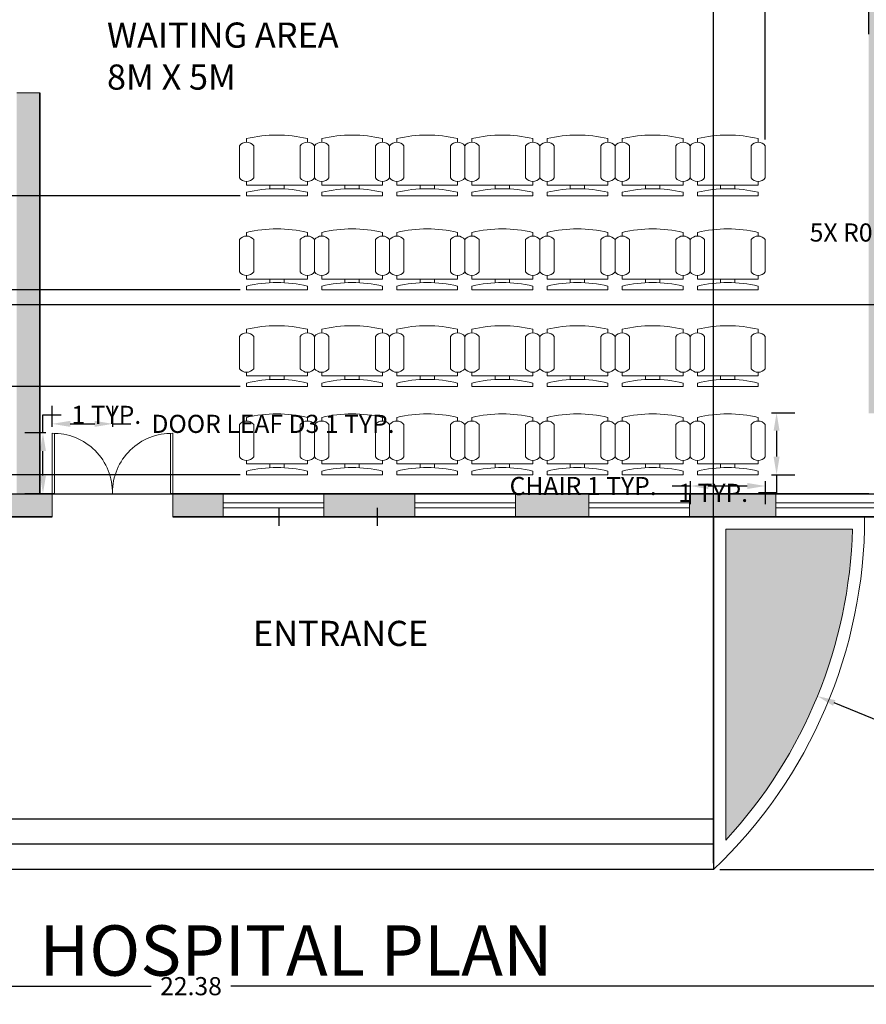
# Model space of a CAD drawing. Units: metres. Extents: x 4298.5 to 4325.2, y 2075 to 2095.8.
# Tile 20 of 35: x 4309.9 to 4318.3, y 2075 to 2084.8. Entities that reach past the tile are written whole.
import ezdxf

# ---------------------------------------------------------------- set-up
doc = ezdxf.new("R2010")
doc.units = ezdxf.units.M
for name, color, linetype, lineweight in [('A-ANNO-DIMS', 2, 'Continuous', 18), ('A-ANNO-TEXT', 7, 'Continuous', 25), ('A-AREA-IDEN', 7, 'Continuous', 18), ('A-DOOR', 3, 'Continuous', 18), ('A-FLOR-STRS', 7, 'Continuous', 25), ('A-FURN', 15, 'Continuous', 18), ('A-GLAZ', 4, 'Continuous', 18), ('A-WALL', 7, 'Continuous', 35), ('A-WALL-PATT', 252, 'Continuous', 13), ('L-PLNT-BEDS', 94, 'Continuous', 18), ('L-PLNT-BEDS-PATT', 252, 'Continuous', 13)]:
    doc.layers.add(name, color=color, linetype=linetype, lineweight=lineweight)
doc.styles.get("Standard").update_dxf_attribs({"font": 'arial.ttf'})
doc.dimstyles.get("Standard").update_dxf_attribs({"dimtxt": 0.18, "dimasz": 0.18, "dimexe": 0.18, "dimexo": 0.0625, "dimgap": 0.09, "dimtad": 0, "dimtih": 1, "dimtoh": 1, "dimdec": 4, "dimzin": 0, "dimdsep": 46, "dimtxsty": 'Standard', "dimcen": 0.09, "dimadec": 0, "dimazin": 0, "dimtfac": 1, "dimtdec": 4, "dimtofl": 0, "dimtmove": 0, "dimatfit": 3, "dimfxl": 1, "dimtolj": 1, "dimtzin": 0, "dimarcsym": 0})

# ---------------------------------------------------------------- blocks, each defined once
blk = doc.blocks.new('Chair - Desk')
for p, q in [((-8.5, 0), (-8.5, -1)), ((-8.5, 0), (8.5, 0)), ((8.5, 0), (8.5, -1)), ((-2, -3), (-2, -1.9355)), ((2, -1.9576), (2, -3)), ((-10.5, -5), (-10.5, -14)), ((-8.5, -3), (-8.5, -4)), ((-8.5, -3), (8.5, -3)), ((-6.5, -14), (-6.5, -5)), ((6.5, -5), (6.5, -14)), ((8.5, -3), (8.5, -4)), ((10.5, -14), (10.5, -5)), ((-8.5, -15), (-8.5, -16)), ((8.5, -15), (8.5, -16))]:
    blk.add_line(p, q)
for centre, radius, start, end in [((0, 34.625), 36.625, 256.5803, 283.4197), ((-8.5, -6.5), 2.5, 36.8699, 143.1301), ((8.5, -6.5), 2.5, 36.8699, 143.1301), ((-8.5, -12.5), 2.5, 216.8699, 323.1301), ((0, 19.625), 36.625, 256.5803, 283.4197), ((8.5, -12.5), 2.5, 216.8699, 323.1301)]:
    blk.add_arc(centre, radius, start, end)
blk = doc.blocks.new('WIN-1000-GLASS')
for p, q in [((1, 0.05), (0, 0.05)), ((1, 0), (0, 0))]:
    blk.add_line(p, q)
blk = doc.blocks.new('DOOR-600-LEAF')
for p, q in [((0, 0), (0, 0.6)), ((0.025, 0), (0.025, 0.6))]:
    blk.add_line(p, q)
blk.add_arc((0.0125, 0.0125), 0.5876, 358.78112, 91.21888)
blk = doc.blocks.new('*D19')
at = {"layer": 'A-ANNO-DIMS', "color": 0, "lineweight": -2, "transparency": 16777216}
for p, q in [((4316.5779, 2080.1351), (4316.3979, 2080.1351)), ((4316.5779, 2080.1845), (4316.5779, 2079.9551)), ((4317.144, 2080.1351), (4316.7579, 2080.1351)), ((4317.324, 2080.1845), (4317.324, 2079.9551))]:
    blk.add_line(p, q, dxfattribs=at)
at = {"layer": 'A-ANNO-DIMS', "color": 0, "transparency": 16777216}
for points in [[(4316.7579, 2080.1651), (4316.7579, 2080.1051), (4316.5779, 2080.1351)], [(4317.144, 2080.1651), (4317.144, 2080.1051), (4317.324, 2080.1351)]]:
    blk.add_solid(points, dxfattribs=at)
at = {"layer": 'Defpoints', "color": 0, "transparency": 16777216}
for p in [(4316.5779, 2080.247), (4317.324, 2080.247), (4316.5779, 2080.1351)]:
    blk.add_point(p, dxfattribs=at)
at = {"layer": 'A-ANNO-DIMS', "color": 0, "transparency": 16777216, "insert": (4315.5147, 2080.1351), "char_height": 0.18, "attachment_point": 5}
blk.add_mtext('\\A1;CHAIR 1 TYP.', dxfattribs=at)
blk = doc.blocks.new('*D20')
at = {"layer": 'A-ANNO-DIMS', "color": 0, "lineweight": -2, "transparency": 16777216}
for p, q in [((4317.3865, 2080.8629), (4317.616, 2080.8629)), ((4317.436, 2080.6829), (4317.436, 2080.427)), ((4317.3865, 2080.247), (4317.616, 2080.247)), ((4317.436, 2080.247), (4317.436, 2080.067)), ((4317.436, 2080.067), (4317.256, 2080.067))]:
    blk.add_line(p, q, dxfattribs=at)
at = {"layer": 'A-ANNO-DIMS', "color": 0, "transparency": 16777216}
for points in [[(4317.406, 2080.6829), (4317.466, 2080.6829), (4317.436, 2080.8629)], [(4317.406, 2080.427), (4317.466, 2080.427), (4317.436, 2080.247)]]:
    blk.add_solid(points, dxfattribs=at)
at = {"layer": 'Defpoints', "color": 0, "transparency": 16777216}
for p in [(4317.324, 2080.8629), (4317.324, 2080.247), (4317.436, 2080.247)]:
    blk.add_point(p, dxfattribs=at)
at = {"layer": 'A-ANNO-DIMS', "color": 0, "transparency": 16777216, "insert": (4316.8063, 2080.067), "char_height": 0.18, "attachment_point": 5}
blk.add_mtext('\\A1;1 TYP.', dxfattribs=at)
blk = doc.blocks.new('*D39')
at = {"layer": 'A-ANNO-DIMS', "color": 0, "lineweight": -2, "transparency": 16777216}
for p, q in [((4310.2406, 2080.724), (4310.2406, 2080.932)), ((4310.844, 2080.724), (4310.844, 2080.932)), ((4310.4206, 2080.752), (4310.664, 2080.752)), ((4310.844, 2080.752), (4311.024, 2080.752))]:
    blk.add_line(p, q, dxfattribs=at)
at = {"layer": 'A-ANNO-DIMS', "color": 0, "transparency": 16777216}
for points in [[(4310.4206, 2080.782), (4310.4206, 2080.722), (4310.2406, 2080.752)], [(4310.664, 2080.782), (4310.664, 2080.722), (4310.844, 2080.752)]]:
    blk.add_solid(points, dxfattribs=at)
at = {"layer": 'Defpoints', "color": 0, "transparency": 16777216}
for p in [(4310.844, 2080.752), (4310.2406, 2080.6615), (4310.844, 2080.6615)]:
    blk.add_point(p, dxfattribs=at)
at = {"layer": 'A-ANNO-DIMS', "color": 0, "transparency": 16777216, "insert": (4312.4348, 2080.752), "char_height": 0.18, "attachment_point": 5}
blk.add_mtext('\\A1;DOOR LEAF D3 1 TYP.', dxfattribs=at)
blk = doc.blocks.new('*D40')
at = {"layer": 'A-ANNO-DIMS', "color": 0, "lineweight": -2, "transparency": 16777216}
for p, q in [((4310.1501, 2080.6615), (4310.1501, 2080.8415)), ((4310.1501, 2080.8415), (4310.3301, 2080.8415)), ((4310.1781, 2080.6615), (4309.9701, 2080.6615)), ((4310.1501, 2080.2381), (4310.1501, 2080.4815)), ((4310.1781, 2080.0581), (4309.9701, 2080.0581))]:
    blk.add_line(p, q, dxfattribs=at)
at = {"layer": 'A-ANNO-DIMS', "color": 0, "transparency": 16777216}
for points in [[(4310.1201, 2080.4815), (4310.1801, 2080.4815), (4310.1501, 2080.6615)], [(4310.1201, 2080.2381), (4310.1801, 2080.2381), (4310.1501, 2080.0581)]]:
    blk.add_solid(points, dxfattribs=at)
at = {"layer": 'Defpoints', "color": 0, "transparency": 16777216}
for p in [(4310.1501, 2080.6615), (4310.2406, 2080.6615), (4310.2406, 2080.0581)]:
    blk.add_point(p, dxfattribs=at)
at = {"layer": 'A-ANNO-DIMS', "color": 0, "transparency": 16777216, "insert": (4310.7798, 2080.8415), "char_height": 0.18, "attachment_point": 5}
blk.add_mtext('\\A1;1 TYP.', dxfattribs=at)
blk = doc.blocks.new('*D47')
at = {"layer": 'A-ANNO-DIMS', "color": 0, "lineweight": -2, "transparency": 16777216}
for p, q in [((4300.4306, 2084.4956), (4300.4306, 2074.9896)), ((4322.8106, 2084.4956), (4322.8106, 2074.9896)), ((4300.6106, 2075.1696), (4311.2252, 2075.1696)), ((4322.6306, 2075.1696), (4312.016, 2075.1696))]:
    blk.add_line(p, q, dxfattribs=at)
at = {"layer": 'A-ANNO-DIMS', "color": 0, "transparency": 16777216}
for points in [[(4300.6106, 2075.1996), (4300.6106, 2075.1396), (4300.4306, 2075.1696)], [(4322.6306, 2075.1996), (4322.6306, 2075.1396), (4322.8106, 2075.1696)]]:
    blk.add_solid(points, dxfattribs=at)
at = {"layer": 'Defpoints', "color": 0, "transparency": 16777216}
for p in [(4300.4306, 2084.5581), (4322.8106, 2084.5581), (4322.8106, 2075.1696)]:
    blk.add_point(p, dxfattribs=at)
at = {"layer": 'A-ANNO-DIMS', "color": 0, "transparency": 16777216, "insert": (4311.6206, 2075.1696), "char_height": 0.18, "attachment_point": 5}
blk.add_mtext('\\A1;22.38', dxfattribs=at)
blk = doc.blocks.new('*D48')
at = {"layer": 'A-ANNO-DIMS', "color": 0, "lineweight": -2, "transparency": 16777216}
for p, q in [((4310.1831, 2094.4781), (4324.7671, 2094.4781)), ((4324.5871, 2094.2981), (4324.5871, 2085.585)), ((4324.5871, 2076.5081), (4324.5871, 2085.2212)), ((4316.8731, 2076.3281), (4324.7671, 2076.3281))]:
    blk.add_line(p, q, dxfattribs=at)
at = {"layer": 'A-ANNO-DIMS', "color": 0, "transparency": 16777216}
for points in [[(4324.5571, 2094.2981), (4324.6171, 2094.2981), (4324.5871, 2094.4781)], [(4324.5571, 2076.5081), (4324.6171, 2076.5081), (4324.5871, 2076.3281)]]:
    blk.add_solid(points, dxfattribs=at)
at = {"layer": 'Defpoints', "color": 0, "transparency": 16777216}
for p in [(4310.1206, 2094.4781), (4316.8106, 2076.3281), (4324.5871, 2076.3281)]:
    blk.add_point(p, dxfattribs=at)
at = {"layer": 'A-ANNO-DIMS', "color": 0, "transparency": 16777216, "insert": (4324.5871, 2085.4031), "char_height": 0.18, "attachment_point": 5}
blk.add_mtext('\\A1;18.15', dxfattribs=at)
blk = doc.blocks.new('*D53')
at = {"layer": 'A-ANNO-DIMS', "color": 0, "lineweight": -2, "transparency": 16777216}
for p, q in [((4309.1606, 2076.3906), (4309.1606, 2095.8166)), ((4316.8106, 2076.3906), (4316.8106, 2095.8166)), ((4309.3406, 2095.6366), (4312.6619, 2095.6366)), ((4316.6306, 2095.6366), (4313.3093, 2095.6366))]:
    blk.add_line(p, q, dxfattribs=at)
at = {"layer": 'A-ANNO-DIMS', "color": 0, "transparency": 16777216}
for points in [[(4309.3406, 2095.6666), (4309.3406, 2095.6066), (4309.1606, 2095.6366)], [(4316.6306, 2095.6666), (4316.6306, 2095.6066), (4316.8106, 2095.6366)]]:
    blk.add_solid(points, dxfattribs=at)
at = {"layer": 'Defpoints', "color": 0, "transparency": 16777216}
for p in [(4316.8106, 2095.6366), (4309.1606, 2076.3281), (4316.8106, 2076.3281)]:
    blk.add_point(p, dxfattribs=at)
at = {"layer": 'A-ANNO-DIMS', "color": 0, "transparency": 16777216, "insert": (4312.9856, 2095.6366), "char_height": 0.18, "attachment_point": 5}
blk.add_mtext('\\A1;7.65', dxfattribs=at)
blk = doc.blocks.new('*D60')
at = {"layer": 'A-ANNO-DIMS', "color": 0, "lineweight": -2, "transparency": 16777216}
for p, q in [((4305.9531, 2081.9381), (4324.7671, 2081.9381)), ((4324.5871, 2081.7581), (4324.5871, 2081.18)), ((4324.5871, 2080.2381), (4324.5871, 2080.8162)), ((4305.9531, 2080.0581), (4324.7671, 2080.0581))]:
    blk.add_line(p, q, dxfattribs=at)
at = {"layer": 'A-ANNO-DIMS', "color": 0, "transparency": 16777216}
for points in [[(4324.5571, 2081.7581), (4324.6171, 2081.7581), (4324.5871, 2081.9381)], [(4324.5571, 2080.2381), (4324.6171, 2080.2381), (4324.5871, 2080.0581)]]:
    blk.add_solid(points, dxfattribs=at)
at = {"layer": 'Defpoints', "color": 0, "transparency": 16777216}
for p in [(4305.8906, 2081.9381), (4324.5871, 2081.9381), (4305.8906, 2080.0581)]:
    blk.add_point(p, dxfattribs=at)
at = {"layer": 'A-ANNO-DIMS', "color": 0, "transparency": 16777216, "insert": (4324.5871, 2080.9981), "char_height": 0.18, "attachment_point": 5}
blk.add_mtext('\\A1;1.88', dxfattribs=at)
blk = doc.blocks.new('*D61')
at = {"layer": 'A-ANNO-DIMS', "color": 0, "lineweight": -2, "transparency": 16777216}
for p, q in [((4317.324045, 2083.575187), (4317.324045, 2095.816556)), ((4318.350577, 2084.620556), (4318.350577, 2095.816556)), ((4317.144045, 2095.636556), (4316.964045, 2095.636556)), ((4318.530577, 2095.636556), (4318.710577, 2095.636556))]:
    blk.add_line(p, q, dxfattribs=at)
at = {"layer": 'A-ANNO-DIMS', "color": 0, "transparency": 16777216}
for points in [[(4317.144045, 2095.666556), (4317.144045, 2095.606556), (4317.324045, 2095.636556)], [(4318.530577, 2095.666556), (4318.530577, 2095.606556), (4318.350577, 2095.636556)]]:
    blk.add_solid(points, dxfattribs=at)
at = {"layer": 'Defpoints', "color": 0, "transparency": 16777216}
for p in [(4318.350577, 2095.636556), (4318.350577, 2084.558056), (4317.324045, 2083.512687)]:
    blk.add_point(p, dxfattribs=at)
at = {"layer": 'A-ANNO-DIMS', "color": 0, "transparency": 16777216, "insert": (4317.837311, 2095.636556), "char_height": 0.18, "attachment_point": 5}
blk.add_mtext('\\A1;1.03', dxfattribs=at)
blk = doc.blocks.new('*D62')
at = {"layer": 'A-ANNO-DIMS', "color": 0, "lineweight": -2, "transparency": 16777216}
for p, q in [((4312.1097, 2083.0153), (4299.0921, 2083.0153)), ((4299.2721, 2082.8353), (4299.2721, 2082.7313)), ((4299.2721, 2082.2635), (4299.2721, 2082.3674)), ((4312.1097, 2082.0835), (4299.0921, 2082.0835))]:
    blk.add_line(p, q, dxfattribs=at)
at = {"layer": 'A-ANNO-DIMS', "color": 0, "transparency": 16777216}
for points in [[(4299.2421, 2082.8353), (4299.3021, 2082.8353), (4299.2721, 2083.0153)], [(4299.2421, 2082.2635), (4299.3021, 2082.2635), (4299.2721, 2082.0835)]]:
    blk.add_solid(points, dxfattribs=at)
at = {"layer": 'Defpoints', "color": 0, "transparency": 16777216}
for p in [(4312.1722, 2083.0153), (4299.2721, 2082.0835), (4312.1722, 2082.0835)]:
    blk.add_point(p, dxfattribs=at)
at = {"layer": 'A-ANNO-DIMS', "color": 0, "transparency": 16777216, "insert": (4299.2721, 2082.5494), "char_height": 0.18, "attachment_point": 5}
blk.add_mtext('\\A1;0.93', dxfattribs=at)
blk = doc.blocks.new('*D63')
at = {"layer": 'A-ANNO-DIMS', "color": 0, "lineweight": -2, "transparency": 16777216}
for p, q in [((4312.1097, 2082.0835), (4299.0921, 2082.0835)), ((4299.2721, 2081.9035), (4299.2721, 2081.7847)), ((4299.2721, 2081.3021), (4299.2721, 2081.4209)), ((4312.1097, 2081.1221), (4299.0921, 2081.1221))]:
    blk.add_line(p, q, dxfattribs=at)
at = {"layer": 'A-ANNO-DIMS', "color": 0, "transparency": 16777216}
for points in [[(4299.2421, 2081.9035), (4299.3021, 2081.9035), (4299.2721, 2082.0835)], [(4299.2421, 2081.3021), (4299.3021, 2081.3021), (4299.2721, 2081.1221)]]:
    blk.add_solid(points, dxfattribs=at)
at = {"layer": 'Defpoints', "color": 0, "transparency": 16777216}
for p in [(4312.1722, 2082.0835), (4299.2721, 2081.1221), (4312.1722, 2081.1221)]:
    blk.add_point(p, dxfattribs=at)
at = {"layer": 'A-ANNO-DIMS', "color": 0, "transparency": 16777216, "insert": (4299.2721, 2081.6028), "char_height": 0.18, "attachment_point": 5}
blk.add_mtext('\\A1;0.96', dxfattribs=at)
blk = doc.blocks.new('*D64')
at = {"layer": 'A-ANNO-DIMS', "color": 0, "lineweight": -2, "transparency": 16777216}
for p, q in [((4312.1097, 2081.1221), (4299.0921, 2081.1221)), ((4299.2721, 2080.9421), (4299.2721, 2080.427)), ((4312.1097, 2080.247), (4299.0921, 2080.247)), ((4299.2721, 2080.247), (4299.2721, 2080.067)), ((4299.2721, 2080.067), (4299.0921, 2080.067))]:
    blk.add_line(p, q, dxfattribs=at)
at = {"layer": 'A-ANNO-DIMS', "color": 0, "transparency": 16777216}
for points in [[(4299.2421, 2080.9421), (4299.3021, 2080.9421), (4299.2721, 2081.1221)], [(4299.2421, 2080.427), (4299.3021, 2080.427), (4299.2721, 2080.247)]]:
    blk.add_solid(points, dxfattribs=at)
at = {"layer": 'Defpoints', "color": 0, "transparency": 16777216}
for p in [(4312.1722, 2081.1221), (4299.2721, 2080.247), (4312.1722, 2080.247)]:
    blk.add_point(p, dxfattribs=at)
at = {"layer": 'A-ANNO-DIMS', "color": 0, "transparency": 16777216, "insert": (4298.7681, 2080.067), "char_height": 0.18, "attachment_point": 5}
blk.add_mtext('\\A1;0.88', dxfattribs=at)
blk = doc.blocks.new('*D78')
at = {"layer": 'A-ANNO-DIMS', "color": 0, "lineweight": -2, "transparency": 16777216}
for p, q in [((4312.4969, 2079.7393), (4312.4969, 2079.9193)), ((4312.4069, 2079.8293), (4312.5869, 2079.8293)), ((4305.3847, 2076.7806), (4307.8863, 2077.853)), ((4305.2047, 2076.7806), (4305.3847, 2076.7806))]:
    blk.add_line(p, q, dxfattribs=at)
at = {"layer": 'A-ANNO-DIMS', "color": 0, "transparency": 16777216}
blk.add_solid([(4307.8745, 2077.8806), (4307.8981, 2077.8254), (4308.0518, 2077.9239)], dxfattribs=at)
at = {"layer": 'Defpoints', "color": 0, "transparency": 16777216}
for p in [(4312.4969, 2079.8293), (4308.0518, 2077.9239)]:
    blk.add_point(p, dxfattribs=at)
at = {"layer": 'A-ANNO-DIMS', "color": 0, "transparency": 16777216, "insert": (4304.53, 2076.7806), "char_height": 0.18, "attachment_point": 5}
blk.add_mtext('\\A1;2X R4.836', dxfattribs=at)
blk = doc.blocks.new('*D79')
at = {"layer": 'A-ANNO-DIMS', "color": 0, "lineweight": -2, "transparency": 16777216}
for p, q in [((4313.4743, 2079.7393), (4313.4743, 2079.9193)), ((4313.3843, 2079.8293), (4313.5643, 2079.8293)), ((4320.4622, 2076.981), (4318.0084, 2077.9812)), ((4320.6422, 2076.981), (4320.4622, 2076.981))]:
    blk.add_line(p, q, dxfattribs=at)
at = {"layer": 'A-ANNO-DIMS', "color": 0, "transparency": 16777216}
blk.add_solid([(4318.0197, 2078.009), (4317.9971, 2077.9534), (4317.8417, 2078.0491)], dxfattribs=at)
at = {"layer": 'Defpoints', "color": 0, "transparency": 16777216}
for p in [(4313.4743, 2079.8293), (4317.8417, 2078.0491)]:
    blk.add_point(p, dxfattribs=at)
at = {"layer": 'A-ANNO-DIMS', "color": 0, "transparency": 16777216, "insert": (4321.3169, 2076.981), "char_height": 0.18, "attachment_point": 5}
blk.add_mtext('\\A1;2X R4.716', dxfattribs=at)
blk = doc.blocks.new('*D81')
at = {"layer": 'A-ANNO-DIMS', "color": 0, "lineweight": -2, "transparency": 16777216}
for p, q in [((4319.9481, 2082.4806), (4319.9481, 2082.6606)), ((4318.8509, 2082.6518), (4319.0828, 2082.6346)), ((4319.8581, 2082.5706), (4320.0381, 2082.5706))]:
    blk.add_line(p, q, dxfattribs=at)
at = {"layer": 'A-ANNO-DIMS', "color": 0, "transparency": 16777216}
blk.add_solid([(4319.085, 2082.6645), (4319.0806, 2082.6047), (4319.2623, 2082.6213)], dxfattribs=at)
at = {"layer": 'Defpoints', "color": 0, "transparency": 16777216}
for p in [(4319.2623, 2082.6213), (4319.9481, 2082.5706)]:
    blk.add_point(p, dxfattribs=at)
at = {"layer": 'A-ANNO-DIMS', "color": 0, "transparency": 16777216, "insert": (4318.2474, 2082.6518), "char_height": 0.18, "attachment_point": 5}
blk.add_mtext('\\A1;5X R0.69', dxfattribs=at)

msp = doc.modelspace()

# ---------------------------------------------------------------- hatches: boundary and pattern name
at = {"layer": 'A-WALL-PATT'}
h = msp.add_hatch(color=256, dxfattribs=at)
h.dxf.hatch_style = 1
h.paths.add_polyline_path([(4308.7606, 2094.4781), (4308.1606, 2094.4781), (4307.4606, 2094.4781), (4307.4606, 2094.2481), (4308.2706, 2094.2481), (4308.2706, 2094.1281), (4308.3906, 2094.1281), (4308.3906, 2094.2481), (4308.7606, 2094.2481)])
h.paths.add_polyline_path([(4310.1206, 2094.4781), (4309.5206, 2094.4781), (4309.5206, 2094.2481), (4309.8906, 2094.2481), (4309.8906, 2092.2481), (4308.3906, 2092.2481), (4308.3906, 2093.4281), (4308.2706, 2093.4281), (4308.2706, 2092.0181), (4309.8906, 2092.0181), (4309.8906, 2087.0181), (4309.7706, 2087.0181), (4309.7706, 2086.7881), (4309.8906, 2086.7881), (4311.9406, 2086.7881), (4311.9406, 2087.0181), (4310.1206, 2087.0181), (4310.1206, 2089.0181), (4310.2406, 2089.0181), (4310.2406, 2089.1381), (4310.1206, 2089.1381), (4310.1206, 2092.0181), (4310.3078, 2092.0181), (4310.3078, 2092.2481), (4310.1206, 2092.2481)])
h.paths.add_polyline_path([(4311.7406, 2092.2481), (4311.0678, 2092.2481), (4311.0678, 2092.0181), (4311.7406, 2092.0181)], flags=17)
h.paths.add_polyline_path([(4313.1733, 2092.2481), (4312.5006, 2092.2481), (4312.5006, 2092.0181), (4313.1733, 2092.0181)])
h.paths.add_polyline_path([(4314.5378, 2092.2481), (4314.1206, 2092.2481), (4313.9333, 2092.2481), (4313.9333, 2092.0181), (4314.1206, 2092.0181), (4314.1206, 2087.0181), (4314.0006, 2087.0181), (4314.0006, 2086.7881), (4314.1206, 2086.7881), (4315.5718, 2086.7881), (4315.5718, 2087.0181), (4314.3506, 2087.0181), (4314.3506, 2092.0181), (4314.5378, 2092.0181)])
h.paths.add_polyline_path([(4315.9706, 2092.2481), (4315.2978, 2092.2481), (4315.2978, 2092.0181), (4315.9706, 2092.0181)])
h.paths.add_polyline_path([(4317.4033, 2092.2481), (4316.7306, 2092.2481), (4316.7306, 2092.0181), (4317.4033, 2092.0181)])
h.paths.add_polyline_path([(4318.9506, 2092.2481), (4318.3506, 2092.2481), (4318.1633, 2092.2481), (4318.1633, 2092.0181), (4318.3506, 2092.0181), (4318.3506, 2091.8981), (4318.5806, 2091.8981), (4318.5806, 2092.0181), (4318.9506, 2092.0181)])
h.paths.add_polyline_path([(4321.0106, 2092.2481), (4319.7106, 2092.2481), (4319.7106, 2092.0181), (4320.0806, 2092.0181), (4320.0806, 2090.0181), (4318.5806, 2090.0181), (4318.5806, 2091.1981), (4318.3506, 2091.1981), (4318.3506, 2090.0181), (4318.3506, 2087.0181), (4318.2306, 2087.0181), (4318.2306, 2086.7881), (4318.3506, 2086.7881), (4318.3506, 2086.3081), (4318.5806, 2086.3081), (4318.5806, 2089.7881), (4321.7806, 2089.7881), (4321.7806, 2090.0181), (4320.2006, 2090.0181), (4320.2006, 2092.0181), (4321.0106, 2092.0181)])
h.paths.add_polyline_path([(4322.8106, 2092.2481), (4321.7706, 2092.2481), (4321.7706, 2092.0181), (4322.5806, 2092.0181), (4322.5806, 2091.2831), (4322.8106, 2091.2831)])
h.paths.add_polyline_path([(4322.8106, 2090.5231), (4322.5806, 2090.5231), (4322.5806, 2089.7881), (4322.5806, 2089.5254), (4322.8106, 2089.5254), (4322.8106, 2090.0181)])
h.paths.add_polyline_path([(4322.8106, 2088.7654), (4322.5806, 2088.7654), (4322.5806, 2087.6681), (4322.8106, 2087.6681)])
h.paths.add_polyline_path([(4322.8106, 2086.9081), (4322.5806, 2086.9081), (4322.5806, 2085.8107), (4322.8106, 2085.8107)])
h.paths.add_polyline_path([(4322.8106, 2085.0507), (4322.5806, 2085.0507), (4322.5806, 2084.7881), (4318.5806, 2084.7881), (4318.5806, 2085.0581), (4318.5806, 2085.4081), (4318.3506, 2085.4081), (4318.3506, 2084.5581), (4318.3506, 2080.8581), (4318.4706, 2080.8581), (4318.4706, 2082.3281), (4319.2606, 2082.3281), (4319.2606, 2082.5581), (4318.5806, 2082.5581), (4318.5806, 2084.5581), (4320.0806, 2084.5581), (4320.0806, 2083.9381), (4320.3106, 2083.9381), (4320.3106, 2084.5581), (4322.8106, 2084.5581)])
h.paths.add_polyline_path([(4320.3106, 2083.1781), (4320.0806, 2083.1781), (4320.0806, 2082.5581), (4319.9606, 2082.5581), (4319.9606, 2082.3281), (4320.0806, 2082.3281), (4320.0806, 2081.5731), (4320.3106, 2081.5731)], flags=17)
h.paths.add_polyline_path([(4320.3106, 2080.8131), (4320.0806, 2080.8131), (4320.0806, 2080.0581), (4318.4286, 2080.0581), (4318.4286, 2079.8281), (4320.3106, 2079.8281)])
h.paths.add_polyline_path([(4317.3506, 2085.2881), (4316.5718, 2085.2881), (4316.5718, 2085.0581), (4317.3506, 2085.0581)])
h.paths.add_polyline_path([(4315.5718, 2085.2881), (4314.8434, 2085.2881), (4314.8434, 2085.0581), (4315.5718, 2085.0581)])
h.paths.add_polyline_path([(4313.8434, 2085.2881), (4312.9406, 2085.2881), (4312.9406, 2085.0581), (4313.8434, 2085.0581)])
h.paths.add_polyline_path([(4311.9406, 2085.2881), (4311.4406, 2085.2881), (4311.4406, 2085.0581), (4311.9406, 2085.0581)])
h.paths.add_polyline_path([(4317.3306, 2087.0181), (4316.5718, 2087.0181), (4316.5718, 2086.7881), (4317.3306, 2086.7881)])
h.paths.add_polyline_path([(4313.1006, 2089.1381), (4311.1406, 2089.1381), (4311.1406, 2089.0181), (4312.9806, 2089.0181), (4312.9806, 2087.0181), (4312.9406, 2087.0181), (4312.9406, 2086.7881), (4313.1006, 2086.7881), (4313.1006, 2087.0181)])
h.paths.add_polyline_path([(4307.5515, 2087.0181), (4305.8906, 2087.0181), (4305.8906, 2092.2481), (4305.8906, 2094.2481), (4306.7006, 2094.2481), (4306.7006, 2094.4781), (4305.6606, 2094.4781), (4305.6606, 2092.2481), (4305.2906, 2092.2481), (4305.2906, 2092.0181), (4305.6606, 2092.0181), (4305.6606, 2090.0181), (4304.1606, 2090.0181), (4304.1606, 2091.1981), (4304.0406, 2091.1981), (4304.0406, 2089.9081), (4301.5606, 2089.9081), (4301.5606, 2089.7881), (4304.0406, 2089.7881), (4305.6606, 2089.7881), (4305.6606, 2086.6381), (4305.8906, 2086.6381), (4305.8906, 2086.7881), (4307.5515, 2086.7881)])
h.paths.add_polyline_path([(4307.5515, 2085.2881), (4305.8906, 2085.2881), (4305.8906, 2085.4381), (4305.6606, 2085.4381), (4305.6606, 2084.7881), (4305.2906, 2084.7881), (4305.2906, 2084.5581), (4305.6606, 2084.5581), (4305.6606, 2084.02), (4305.8906, 2084.02), (4305.8906, 2084.5581), (4305.8906, 2085.0581), (4307.5515, 2085.0581)])
h.paths.add_polyline_path([(4310.2406, 2085.2881), (4308.5515, 2085.2881), (4308.5515, 2085.0581), (4310.2406, 2085.0581)])
h.paths.add_polyline_path([(4317.4286, 2080.0581), (4316.5718, 2080.0581), (4316.5718, 2079.8281), (4317.4286, 2079.8281)])
h.paths.add_polyline_path([(4315.5718, 2080.0581), (4314.8434, 2080.0581), (4314.8434, 2079.8281), (4315.5718, 2079.8281)])
h.paths.add_polyline_path([(4313.8434, 2080.0581), (4312.9406, 2080.0581), (4312.9406, 2079.8281), (4313.8434, 2079.8281)])
h.paths.add_polyline_path([(4311.9406, 2080.0581), (4311.4406, 2080.0581), (4311.4406, 2079.8281), (4311.9406, 2079.8281)])
h.paths.add_polyline_path([(4310.2406, 2080.0581), (4310.1206, 2080.0581), (4310.1206, 2084.0381), (4309.8906, 2084.0381), (4309.8906, 2080.0581), (4309.1606, 2080.0581), (4309.1606, 2079.8281), (4310.2406, 2079.8281)])
h.paths.add_polyline_path([(4308.1606, 2080.0581), (4307.5106, 2080.0581), (4307.5106, 2080.1781), (4307.3906, 2080.1781), (4307.3906, 2080.0581), (4305.8906, 2080.0581), (4305.8906, 2080.567), (4305.6606, 2080.567), (4305.6606, 2079.8281), (4308.1606, 2079.8281)])
h.paths.add_polyline_path([(4307.5106, 2081.9381), (4309.0906, 2081.9381), (4309.0906, 2082.0581), (4305.8906, 2082.0581), (4305.8906, 2083.26), (4305.6606, 2083.26), (4305.6606, 2081.327), (4305.8906, 2081.327), (4305.8906, 2081.9381), (4307.3906, 2081.9381), (4307.3906, 2080.8781), (4307.5106, 2080.8781)])
h.paths.add_polyline_path([(4304.5306, 2084.7881), (4302.7306, 2084.7881), (4302.7306, 2084.5581), (4304.5306, 2084.5581)])
h.paths.add_polyline_path([(4301.9706, 2084.7881), (4300.6606, 2084.7881), (4300.6606, 2085.0249), (4300.4306, 2085.0249), (4300.4306, 2084.5581), (4301.9706, 2084.5581)])
h.paths.add_polyline_path([(4300.6606, 2086.8843), (4300.4306, 2086.8843), (4300.4306, 2085.7849), (4300.6606, 2085.7849)])
h.paths.add_polyline_path([(4300.6606, 2089.1618), (4300.4306, 2089.1618), (4300.4306, 2087.6443), (4300.6606, 2087.6443)])
h.paths.add_polyline_path([(4300.6606, 2091.0212), (4300.4306, 2091.0212), (4300.4306, 2089.9218), (4300.6606, 2089.9218)])
h.paths.add_polyline_path([(4300.6606, 2092.0181), (4301.9706, 2092.0181), (4301.9706, 2092.2481), (4300.4306, 2092.2481), (4300.4306, 2091.7812), (4300.6606, 2091.7812)])
h.paths.add_polyline_path([(4304.5306, 2092.2481), (4302.7306, 2092.2481), (4302.7306, 2092.0181), (4304.0406, 2092.0181), (4304.0406, 2091.8981), (4304.1606, 2091.8981), (4304.1606, 2092.0181), (4304.5306, 2092.0181)], flags=17)
at = {"layer": 'L-PLNT-BEDS-PATT'}
h = msp.add_hatch(dxfattribs=at)
h.set_pattern_fill('TRIANG', color=256, scale=0.02)
h.paths.add_polyline_path([(4309.0406, 2079.7081), (4307.7821, 2079.7081, 0.182638), (4309.0406, 2076.6204)])
h.paths.add_polyline_path([(4318.189, 2079.7081), (4316.9306, 2079.7081), (4316.9306, 2076.6204, 0.182638)])

# ---------------------------------------------------------------- linework, layer by layer
at = {"layer": 'A-DOOR'}
for p, q in [((4309.8906, 2084.0381), (4310.1206, 2084.0381)), ((4311.4156, 2080.0581), (4311.4156, 2080.6581)), ((4311.4406, 2080.0581), (4311.4406, 2080.6581)), ((4310.2406, 2080.0581), (4310.2406, 2079.8281)), ((4311.4406, 2080.0581), (4311.4406, 2079.8281))]:
    msp.add_line(p, q, dxfattribs=at)
msp.add_arc((4311.4281, 2080.0708), 0.5874, 88.78057, 180.02594, dxfattribs=at)
at = {"layer": 'A-FLOR-STRS'}
for p, q in [((4316.8106, 2079.8281), (4316.8106, 2076.3281)), ((4316.8106, 2076.8281), (4309.1606, 2076.8281)), ((4316.8106, 2076.5781), (4309.1606, 2076.5781)), ((4316.8106, 2076.3281), (4309.1606, 2076.3281))]:
    msp.add_line(p, q, dxfattribs=at)
at = {"layer": 'A-GLAZ'}
for p, q in [((4311.9406, 2080.0581), (4311.9406, 2079.8281)), ((4312.9406, 2079.8281), (4312.9406, 2080.0581)), ((4313.8434, 2079.8281), (4313.8434, 2080.0581)), ((4314.8434, 2079.8281), (4314.8434, 2080.0581)), ((4315.5718, 2079.8281), (4315.5718, 2080.0581)), ((4316.5718, 2079.8281), (4316.5718, 2080.0581)), ((4317.4286, 2079.8281), (4317.4286, 2080.0581))]:
    msp.add_line(p, q, dxfattribs=at)
at = {"layer": 'A-WALL'}
for p, q in [((4310.1206, 2084.0381), (4310.1206, 2080.0581)), ((4310.2656, 2080.0581), (4310.1206, 2080.0581)), ((4318.3506, 2080.0581), (4311.4156, 2080.0581)), ((4310.2406, 2079.8281), (4305.6606, 2079.8281)), ((4320.3106, 2079.8281), (4311.4406, 2079.8281))]:
    msp.add_line(p, q, dxfattribs=at)
at = {"layer": 'L-PLNT-BEDS'}
for q in [(4318.189, 2079.7081), (4316.9306, 2076.6204)]:
    msp.add_line((4316.9306, 2079.7081), q, dxfattribs=at)
for radius, start, end in [(4.8363, 313.61799, 359.98483), (4.7163, 317.12523, 358.52647)]:
    msp.add_arc((4313.4743, 2079.8293), radius, start, end, dxfattribs=at)

# ---------------------------------------------------------------- block references
at = {"layer": 'A-DOOR'}
msp.add_blockref('DOOR-600-LEAF', (4310.2406, 2080.0581), dxfattribs=at)
at = {"layer": 'A-FURN', "xscale": 0.035529987753355, "yscale": 0.035529987753355, "zscale": 0.035529987753355, "rotation": 180}
for p in [(4312.4742, 2083.0153), (4313.2203, 2083.0153), (4313.9665, 2083.0153), (4314.7126, 2083.0153), (4315.4587, 2083.0153), (4316.2049, 2083.0153), (4316.951, 2083.0153), (4312.4742, 2082.0835), (4313.2203, 2082.0835), (4313.9665, 2082.0835), (4314.7126, 2082.0835), (4315.4587, 2082.0835), (4316.2049, 2082.0835), (4316.951, 2082.0835), (4312.4742, 2081.1221), (4313.2203, 2081.1221), (4313.9665, 2081.1221), (4314.7126, 2081.1221), (4315.4587, 2081.1221), (4316.2049, 2081.1221), (4316.951, 2081.1221), (4312.4742, 2080.247), (4313.2203, 2080.247), (4313.9665, 2080.247), (4314.7126, 2080.247), (4315.4587, 2080.247), (4316.2049, 2080.247), (4316.951, 2080.247)]:
    msp.add_blockref('Chair - Desk', p, dxfattribs=at)
at = {"layer": 'A-GLAZ', "rotation": 180}
for p in [(4312.9406, 2079.9681), (4314.8434, 2079.9681), (4316.5718, 2079.9681)]:
    msp.add_blockref('WIN-1000-GLASS', p, dxfattribs=at)
at = {"layer": 'A-GLAZ'}
msp.add_blockref('WIN-1000-GLASS', (4317.4286, 2079.9181), dxfattribs=at)

# ---------------------------------------------------------------- texts
at = {"layer": 'A-ANNO-TEXT', "insert": (4310.1143, 2075.7734), "char_height": 0.5, "attachment_point": 1}
msp.add_mtext_dynamic_manual_height_columns('{\\fArial|b1|i0|c0|p34;HOSPITAL PLAN}', width=10.15538, gutter_width=12.5, heights=[0], dxfattribs=at)
at = {"layer": 'A-AREA-IDEN', "char_height": 0.25, "attachment_point": 1}
for s, width, insert in [('WAITING AREA\\P8M X 5M', 4.265171, (4310.7859, 2084.7366)), ('ENTRANCE', 4.559766, (4312.2357, 2078.7968))]:
    msp.add_mtext_dynamic_manual_height_columns(s, width=width, gutter_width=12.5, heights=[0], dxfattribs=dict(at, insert=insert))

# ---------------------------------------------------------------- dimensions: what is measured, and where the dimension line sits
at = {"layer": 'A-ANNO-DIMS'}
for base, p1, p2, picture, middle in [((4316.8106, 2095.6366), (4309.1606, 2076.3281), (4316.8106, 2076.3281), '*D53', (4312.9856, 2095.6366)), ((4318.3506, 2095.6366), (4317.324, 2083.5127), (4318.3506, 2084.5581), '*D61', (4317.8373, 2095.6366)), ((4322.8106, 2075.1696), (4300.4306, 2084.5581), (4322.8106, 2084.5581), '*D47', (4311.6206, 2075.1696))]:
    dim = msp.add_linear_dim(base=base, p1=p1, p2=p2, dimstyle='Standard', override={"dimdec": 2, "dimlfac": 1, "dimrnd": 0, "dimzin": 0, "dimdsep": 46, "dimlunit": 2}, dxfattribs=at)
    dim.commit()
    dim.dimension.update_dxf_attribs({"geometry": picture, "text_midpoint": middle})
for base, p1, p2, picture, middle in [((4324.5871, 2076.3281), (4310.1206, 2094.4781), (4316.8106, 2076.3281), '*D48', (4324.5871, 2085.4031)), ((4299.2721, 2082.0835), (4312.1722, 2083.0153), (4312.1722, 2082.0835), '*D62', (4299.2721, 2082.5494)), ((4299.2721, 2081.1221), (4312.1722, 2082.0835), (4312.1722, 2081.1221), '*D63', (4299.2721, 2081.6028)), ((4324.5871, 2081.9381), (4305.8906, 2080.0581), (4305.8906, 2081.9381), '*D60', (4324.5871, 2080.9981)), ((4299.2721, 2080.247), (4312.1722, 2081.1221), (4312.1722, 2080.247), '*D64', (4298.7681, 2080.067))]:
    dim = msp.add_linear_dim(base=base, p1=p1, p2=p2, angle=90, dimstyle='Standard', override={"dimdec": 2, "dimlfac": 1, "dimrnd": 0, "dimzin": 0, "dimdsep": 46, "dimlunit": 2}, dxfattribs=at)
    dim.commit()
    dim.dimension.update_dxf_attribs({"geometry": picture, "text_midpoint": middle})
for center, mpoint, text, override, picture, middle in [((4319.9481, 2082.5706), (4319.2623, 2082.6213), '5X <>', {"dimdec": 2, "dimlfac": 1, "dimrnd": 0, "dimzin": 0, "dimdsep": 46, "dimlunit": 2}, '*D81', (4318.8509, 2082.6518)), ((4312.4969, 2079.8293), (4308.0518, 2077.9239), '2X <>', {"dimdec": 3, "dimlfac": 1, "dimrnd": 0, "dimzin": 0, "dimdsep": 46, "dimlunit": 2}, '*D78', (4304.53, 2076.7806)), ((4313.4743, 2079.8293), (4317.8417, 2078.0491), '2X <>', {"dimdec": 3, "dimlfac": 1, "dimrnd": 0, "dimzin": 0, "dimdsep": 46, "dimlunit": 2}, '*D79', (4321.3169, 2076.981))]:
    dim = msp.add_radius_dim(center=center, mpoint=mpoint, text=text, dimstyle='Standard', override=override, dxfattribs=at)
    dim.commit()
    dim.dimension.update_dxf_attribs({"geometry": picture, "text_midpoint": middle, "dimtype": 164})
dim = msp.add_linear_dim(base=(4310.844, 2080.752), p1=(4310.2406, 2080.6615), p2=(4310.844, 2080.6615), text='DOOR LEAF D3 <> TYP.', dimstyle='Standard', override={"dimdec": 0, "dimlfac": 1, "dimrnd": 0, "dimzin": 0, "dimdsep": 46, "dimlunit": 2}, dxfattribs=at)
dim.commit()
dim.dimension.update_dxf_attribs({"geometry": '*D39', "text_midpoint": (4312.4348, 2080.752)})
for base, p1, p2, angle, text, picture, middle in [((4310.1501, 2080.6615), (4310.2406, 2080.0581), (4310.2406, 2080.6615), 90, '<> TYP.', '*D40', (4310.7798, 2080.8415)), ((4317.436, 2080.247), (4317.324, 2080.8629), (4317.324, 2080.247), 270, '<> TYP.', '*D20', (4316.8063, 2080.067)), ((4316.5779, 2080.1351), (4317.324, 2080.247), (4316.5779, 2080.247), 180, 'CHAIR <> TYP.', '*D19', (4315.5147, 2080.1351))]:
    dim = msp.add_linear_dim(base=base, p1=p1, p2=p2, angle=angle, text=text, dimstyle='Standard', override={"dimdec": 0, "dimlfac": 1, "dimrnd": 0, "dimzin": 0, "dimdsep": 46, "dimlunit": 2}, dxfattribs=at)
    dim.commit()
    dim.dimension.update_dxf_attribs({"geometry": picture, "text_midpoint": middle})

doc.saveas('drawing.dxf')
